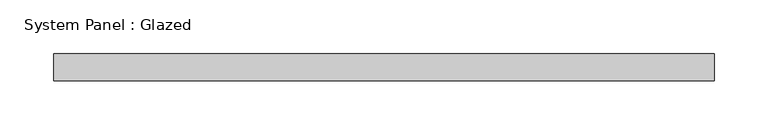
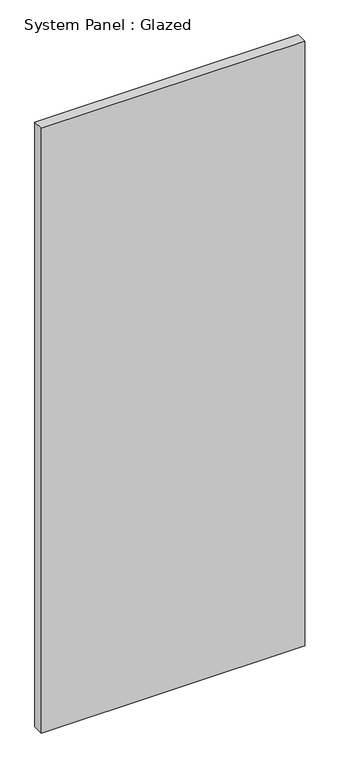
"""IFC4 building model written with IfcOpenShell, lengths in millimetres: plate geometry, System Panel : Glazed."""

from ifc_helpers import new_model, si_unit, origin, origin_with_axes, place, context, project, spatial, polyline, outline, extrude, source, transform, mapped, element, save


def system_panel_glazed_eebfb88d(model_context):
    return source(origin(), model_context, "Body", "SweptSolid", [
        extrude(outline(polyline([(307.975, 19.05), (-307.975, 19.05), (-307.975, 44.45), (307.975, 44.45), (307.975, 19.05)])), origin_with_axes(), (0.0, 0.0, 1.0), 1493.8138027),
    ])


if __name__ == "__main__":
    model = new_model("IFC4")
    model_context = context("Model", 3, world=origin())
    ifc_project = project(units=[si_unit("LENGTHUNIT", "METRE", prefix="MILLI")], contexts=[model_context])
    site = spatial("IfcSite", under=ifc_project)
    building = spatial("IfcBuilding", under=site)
    placement = place(None, origin())
    system_panel_glazed_shape = system_panel_glazed_eebfb88d(model_context)
    element("IfcPlate", 1, ObjectType="System Panel : Glazed", at=placement, inside=building, context=model_context, shape_type="MappedRepresentation", body=[
        mapped(system_panel_glazed_shape, transform((0.0, 0.0, 0.0), x_axis=(1.0, 0.0, 0.0), y_axis=(0.0, 1.0, 0.0), z_axis=(0.0, 0.0, 1.0))),
    ])
    save(model, "model.ifc")

# Revit data of these elements
# Type "System Panel : Glazed"
#   Construction Type Id = "GSP4R"
#   Analytic Construction = "1/8 in Pilkington single glazing"
#   Visual Light Transmittance = 0.9
#   Solar Heat Gain Coefficient = 0.86
#   Heat Transfer Coefficient (U) = 1.18115 BTU/(h·ft²·°F)
#   Define Thermal Properties by = 1
# Element 1 (IfcPlate, "System Panel : Glazed")
#   Materials on its faces: "Glass"
# Materials
#   "Glass": class "Glass", colour RGB 0 128 192, transparency 0.75, Description = "Soda Lime Glass", Cost = 0
